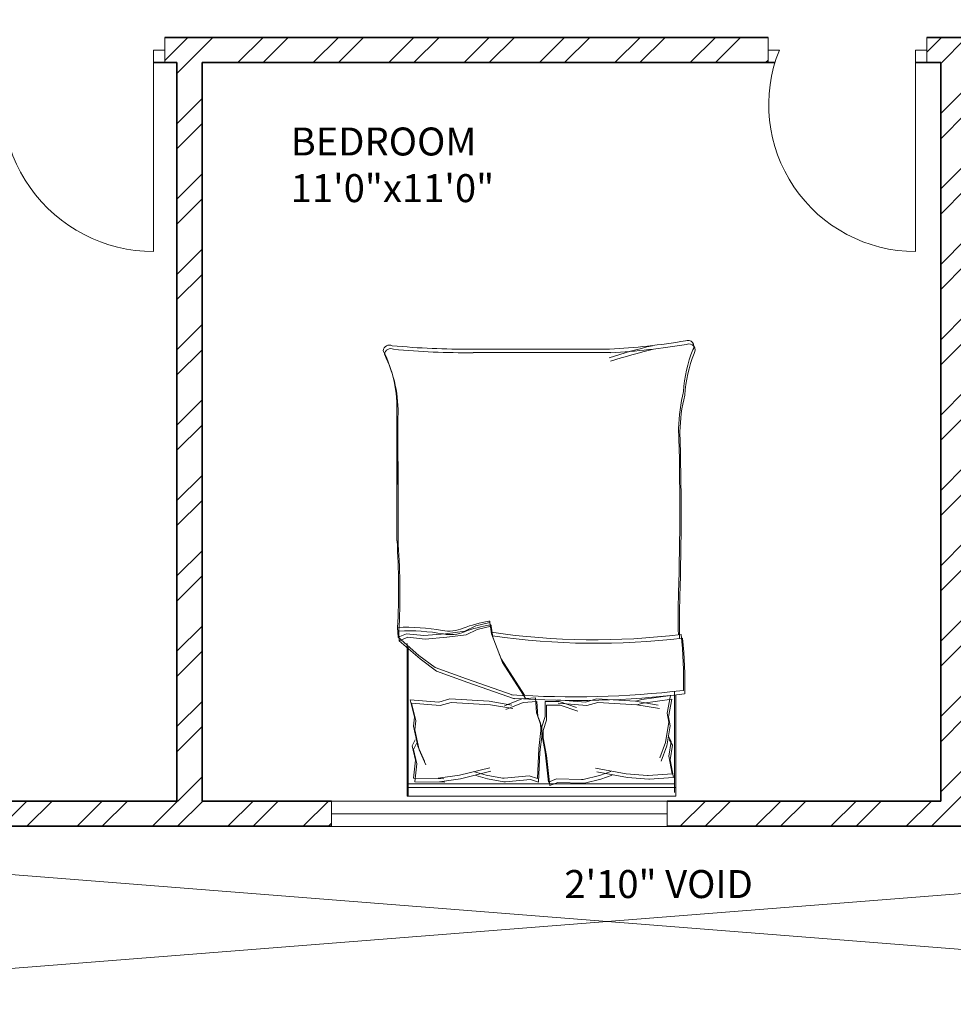
# Model space of a CAD drawing. Units: inches. Extents: x 1885 to 2748, y 783 to 2421.
# Tile 80 of 117: x 2127 to 2294, y 1850 to 2026. Entities that reach past the tile are written whole.
import ezdxf

# ---------------------------------------------------------------- set-up
doc = ezdxf.new("R2010")
doc.units = ezdxf.units.IN
for name, color, linetype, lineweight in [('A-AREA-IDEN', 7, 'Continuous', 18), ('A-DOOR', 31, 'Continuous', 18), ('A-FLOR-OPEN', 8, 'Continuous', 13), ('A-FURN', 8, 'Continuous', 13), ('A-GLAZ', 181, 'Continuous', 18), ('A-WALL', 7, 'Continuous', 35)]:
    doc.layers.add(name, color=color, linetype=linetype, lineweight=lineweight)
doc.layers.add('A-WALL-PATT', color=85, linetype='Continuous', lineweight=13, true_color=0x58ba48)
doc.styles.get("Standard").update_dxf_attribs({"font": 'arial.ttf'})

# ---------------------------------------------------------------- blocks, each defined once
blk = doc.blocks.new('BED-DOUBLE')
for p, q in [((27.75, 52.87), (24.5, 49.16)), ((27.75, 52.87), (24.5, 49.16)), ((28.39, 53.09), (25.14, 49.39)), ((28.39, 53.09), (25.14, 49.39)), ((29.49, 52.95), (27.75, 52.87, 3.87)), ((29.49, 52.95), (27.75, 52.87, 3.87)), ((28.37, 51.33), (27.75, 52.87)), ((28.37, 51.33), (27.75, 52.87)), ((30.13, 53.17), (28.39, 53.09, 3.87)), ((30.13, 53.17), (28.39, 53.09, 3.87)), ((29.01, 51.56), (28.39, 53.09)), ((29.01, 51.56), (28.39, 53.09)), ((0, 51.49), (0.64, 51.49)), ((0, 3.47), (0, 51.49)), ((0, 51.26), (26.61, 51.26)), ((0, 51.26), (26.61, 51.26)), ((0.64, 51.49), (27.25, 51.49)), ((0.64, 51.49), (27.25, 51.49)), ((1.54, 3.47), (1.54, 51.26)), ((1.54, 3.47), (1.54, 51.26)), ((2.18, 3.7), (2.18, 51.49)), ((2.18, 3.7), (2.18, 51.49)), ((28.06, 48.23), (28.37, 51.33)), ((28.06, 48.23), (28.37, 51.33)), ((28.7, 48.46), (29.01, 51.56)), ((28.7, 48.46), (29.01, 51.56)), ((2.56, 50.11), (2.46, 44.71)), ((2.56, 50.11), (2.46, 44.71)), ((2.56, 50.11), (5.77, 49.73)), ((2.56, 50.11), (5.77, 49.73)), ((3.2, 50.34), (3.1, 44.94)), ((3.2, 50.34), (3.1, 44.94)), ((3.2, 50.34), (6.41, 49.96)), ((3.2, 50.34), (6.41, 49.96)), ((8.26, 49.31), (5.58, 48.13)), ((8.26, 49.31), (5.58, 48.13)), ((5.77, 49.73), (8.34, 50.33)), ((5.77, 49.73), (8.34, 50.33)), ((8.9, 49.54), (6.22, 48.36)), ((8.9, 49.54), (6.22, 48.36)), ((6.41, 49.96), (8.98, 50.56)), ((6.41, 49.96), (8.98, 50.56)), ((11.83, 50.11), (8.26, 49.31)), ((11.83, 50.11), (8.26, 49.31)), ((8.34, 50.33), (9.39, 49.81)), ((8.34, 50.33), (9.39, 49.81)), ((12.47, 50.34), (8.9, 49.54)), ((12.47, 50.34), (8.9, 49.54)), ((8.98, 50.56), (10.03, 50.04)), ((8.98, 50.56), (10.03, 50.04)), ((13.44, 49.92), (11.83, 50.11)), ((13.44, 49.92), (11.83, 50.11)), ((14.08, 50.15), (12.47, 50.34)), ((14.08, 50.15), (12.47, 50.34)), ((16.58, 50.7), (13.44, 49.92)), ((16.58, 50.7), (13.44, 49.92)), ((17.22, 50.93), (14.08, 50.15)), ((17.22, 50.93), (14.08, 50.15)), ((16.17, 45.57), (16.58, 50.7)), ((16.17, 45.56), (16.58, 50.7)), ((16.81, 45.79), (17.22, 50.93)), ((16.81, 45.79), (17.22, 50.93)), ((25.14, 49.39), (22.97, 46.45)), ((25.14, 49.39), (22.97, 46.45)), ((24.5, 49.16), (22.33, 46.22)), ((24.5, 49.16), (22.33, 46.22)), ((28.37, 44.36), (28.06, 48.23)), ((28.37, 44.36), (28.06, 48.23)), ((29.01, 44.59), (28.7, 48.46)), ((29.01, 44.59), (28.7, 48.46)), ((3.1, 44.94), (3.19, 45.94)), ((3.1, 44.94), (3.19, 45.94)), ((3.19, 45.94), (3.71, 42.14)), ((3.19, 45.94), (3.71, 42.14)), ((17.37, 43.83), (16.81, 45.79)), ((17.37, 43.83), (16.81, 45.79)), ((22.33, 46.22), (20.32, 40.64)), ((22.33, 46.22), (20.32, 40.64)), ((22.97, 46.45), (20.96, 40.87)), ((22.97, 46.45), (20.96, 40.87)), ((2.46, 44.71), (2.55, 45.71)), ((2.46, 44.71), (2.55, 45.71)), ((2.55, 45.71), (3.07, 41.91)), ((2.55, 45.71), (3.07, 41.91)), ((16.73, 43.6), (16.17, 45.57)), ((16.73, 43.6), (16.17, 45.56)), ((28.83, 40.95), (28.37, 44.36)), ((28.83, 40.95), (28.37, 44.36)), ((29.47, 41.18), (29.01, 44.59)), ((29.47, 41.18), (29.01, 44.59)), ((16.3, 36.59), (16.73, 43.6)), ((16.3, 36.59), (16.73, 43.6)), ((16.94, 36.82), (17.37, 43.83)), ((16.94, 36.82), (17.37, 43.83)), ((3.07, 41.91), (4.43, 36.49)), ((3.07, 41.91), (4.43, 36.49)), ((3.71, 42.14), (5.07, 36.72)), ((3.71, 42.14), (5.07, 36.72)), ((20.32, 40.64), (17.39, 32.3)), ((20.32, 40.64), (17.39, 32.3)), ((20.96, 40.87), (18.03, 32.53)), ((20.96, 40.87), (18.03, 32.53)), ((29.76, 38.94), (28.83, 40.95)), ((29.76, 38.94), (28.83, 40.95)), ((30.4, 39.17), (29.47, 41.18)), ((30.4, 39.17), (29.47, 41.18)), ((3.68, 39.2), (3.08, 37.13)), ((3.68, 39.2), (3.08, 37.13)), ((4.32, 39.43), (3.72, 37.36)), ((4.32, 39.43), (3.72, 37.36)), ((30.38, 36.46), (29.76, 38.94)), ((30.38, 36.46), (29.76, 38.94)), ((31.02, 36.69), (30.4, 39.17)), ((31.02, 36.69), (30.4, 39.17)), ((79.25, 15.06), (79.25, 39.68)), ((79.25, 15.06), (79.25, 39.68)), ((79.89, 15.29), (79.89, 39.9)), ((79.89, 15.29), (79.89, 39.9)), ((3.08, 37.13), (2.54, 34.2)), ((3.08, 37.13), (2.54, 34.2)), ((3.72, 37.36), (3.18, 34.43)), ((3.72, 37.36), (3.18, 34.43)), ((15.63, 32.56), (16.3, 36.59)), ((15.63, 32.56), (16.3, 36.59)), ((16.27, 32.79), (16.94, 36.82)), ((16.27, 32.79), (16.94, 36.82)), ((23.88, 34.45), (28.37, 36.15)), ((23.88, 34.45), (28.37, 36.15)), ((24.52, 34.68), (29.01, 36.38)), ((24.52, 34.68), (29.01, 36.38)), ((28.37, 36.15), (30.38, 36.46)), ((28.37, 36.15), (30.38, 36.46)), ((29.01, 36.38), (31.02, 36.69)), ((29.01, 36.38), (31.02, 36.69)), ((2.54, 34.2), (2.56, 33.88)), ((2.54, 34.2), (2.56, 33.88)), ((2.56, 33.88), (2.98, 29.45)), ((2.56, 33.88), (2.98, 29.45)), ((3.18, 34.43), (3.2, 34.11)), ((3.18, 34.43), (3.2, 34.11)), ((3.2, 34.11), (3.62, 29.68)), ((3.2, 34.11), (3.62, 29.68)), ((16.74, 30.75), (15.46, 33.82)), ((16.74, 30.75), (15.46, 33.82)), ((17.38, 30.98), (16.1, 34.05)), ((17.38, 30.98), (16.1, 34.05)), ((17.39, 30.26), (23.88, 34.45)), ((17.39, 30.26), (23.88, 34.45)), ((18.03, 30.49), (24.52, 34.68)), ((18.03, 30.49), (24.52, 34.68)), ((16.9, 28.3), (16.74, 30.75)), ((16.9, 28.3), (16.74, 30.75)), ((17.54, 28.52), (17.38, 30.98)), ((17.54, 28.52), (17.38, 30.98)), ((2.98, 29.45), (2.5, 27.98)), ((2.98, 29.45), (2.5, 27.98)), ((3.62, 29.68), (3.13, 28.2)), ((3.62, 29.68), (3.13, 28.2)), ((3.13, 28.2), (8.51, 27.96)), ((3.13, 28.2), (8.51, 27.96)), ((13.02, 27.66), (14.86, 28.36)), ((13.02, 27.66), (14.86, 28.36)), ((14.22, 28.13), (16.9, 28.3)), ((14.22, 28.13), (16.9, 28.3)), ((14.86, 28.36), (17.54, 28.52)), ((14.86, 28.36), (17.54, 28.52)), ((1.87, 25.98), (7.22, 26.56)), ((1.87, 25.98), (7.22, 26.56)), ((2.5, 27.98), (7.87, 27.73)), ((2.5, 27.98), (7.87, 27.73)), ((2.51, 26.21), (7.86, 26.79)), ((2.51, 26.21), (7.86, 26.79)), ((7.22, 26.56), (10.4, 27.14)), ((7.22, 26.56), (10.4, 27.14)), ((7.86, 26.79), (11.04, 27.37)), ((7.86, 26.79), (11.04, 27.37)), ((7.87, 27.73), (11.08, 27.35)), ((7.87, 27.73), (11.08, 27.35)), ((8.51, 27.96), (11.72, 27.58)), ((8.51, 27.96), (11.72, 27.58)), ((10.4, 27.14), (11.71, 27.14)), ((10.4, 27.14), (11.71, 27.14)), ((11.04, 27.37), (12.35, 27.37)), ((11.04, 27.37), (12.35, 27.37)), ((11.08, 27.35), (12.38, 27.43)), ((11.08, 27.35), (12.38, 27.43)), ((11.71, 27.14), (13.59, 26.56)), ((11.71, 27.14), (13.59, 26.56)), ((11.72, 27.58), (13.02, 27.66)), ((11.72, 27.58), (13.02, 27.66)), ((12.35, 27.37), (14.22, 26.79)), ((12.35, 27.37), (14.22, 26.79)), ((12.38, 27.43), (14.22, 28.13)), ((12.38, 27.43), (14.22, 28.13)), ((13.59, 26.56), (16.27, 26.56)), ((13.59, 26.56), (16.27, 26.56)), ((14.22, 26.79), (16.91, 26.79)), ((14.22, 26.79), (16.91, 26.79)), ((16.27, 26.56), (16.27, 24.1)), ((16.27, 26.56), (16.27, 24.1)), ((16.91, 26.79), (16.91, 24.33)), ((16.91, 26.79), (16.91, 24.33)), ((2.45, 24.54), (1.87, 25.98)), ((2.45, 24.54), (1.87, 25.98)), ((3.09, 24.76), (2.51, 26.21)), ((3.09, 24.76), (2.51, 26.21)), ((2.95, 20.32), (3.09, 24.76)), ((2.95, 20.32), (3.09, 24.76)), ((16.81, 19.61), (17.22, 24.74)), ((16.81, 19.61), (17.22, 24.74)), ((2.31, 20.09), (2.45, 24.54)), ((2.31, 20.09), (2.45, 24.54)), ((16.27, 24.1), (15.18, 20.96)), ((16.27, 24.1), (15.18, 20.96)), ((16.91, 24.33), (15.82, 21.19)), ((16.91, 24.33), (15.82, 21.19)), ((16.17, 19.38), (16.58, 24.51)), ((16.17, 19.38), (16.58, 24.51)), ((2.31, 19.77), (2.31, 20.09)), ((2.31, 19.77), (2.31, 20.09)), ((3.03, 16.88), (2.31, 19.77)), ((3.03, 16.88), (2.31, 19.77)), ((2.95, 20), (2.95, 20.32)), ((2.95, 20), (2.95, 20.32)), ((3.67, 17.11), (2.95, 20)), ((3.67, 17.11), (2.95, 20)), ((16.73, 17.42), (16.17, 19.38)), ((16.73, 17.42), (16.17, 19.38)), ((17.37, 17.65), (16.81, 19.61)), ((17.37, 17.65), (16.81, 19.61)), ((3.32, 12.11), (4.33, 17.6)), ((3.32, 12.11), (4.33, 17.6)), ((3.96, 12.34), (4.97, 17.83)), ((3.96, 12.34), (4.97, 17.83)), ((16.94, 10.64), (17.37, 17.65)), ((16.94, 10.64), (17.37, 17.65)), ((3.75, 14.85), (3.03, 16.88)), ((3.75, 14.85), (3.03, 16.88)), ((4.39, 15.08), (3.67, 17.11)), ((4.39, 15.08), (3.67, 17.11)), ((16.3, 10.41), (16.73, 17.42)), ((16.3, 10.41), (16.73, 17.42)), ((3.67, 8.51), (3.96, 12.34)), ((3.67, 8.51), (3.96, 12.34)), ((3.03, 8.28), (3.32, 12.11)), ((3.03, 8.28), (3.32, 12.11)), ((16.27, 6.61), (16.94, 10.64)), ((16.27, 6.61), (16.94, 10.64)), ((16.94, 10.64), (17.26, 9.51)), ((16.94, 10.64), (17.26, 9.51)), ((15.63, 6.38), (16.3, 10.41)), ((15.63, 6.38), (16.3, 10.41)), ((16.3, 10.41), (16.62, 9.28)), ((16.3, 10.41), (16.62, 9.28)), ((16.62, 9.28), (17.34, 4.18)), ((16.62, 9.28), (17.34, 4.18)), ((17.26, 9.51), (17.98, 4.41)), ((17.26, 9.51), (17.98, 4.41)), ((3.01, 8.18), (3.03, 8.28)), ((3.01, 8.18), (3.03, 8.28)), ((3.34, 3.9), (3.01, 8.18)), ((3.34, 3.9), (3.01, 8.18)), ((3.65, 8.41), (3.67, 8.51)), ((3.65, 8.41), (3.67, 8.51)), ((3.98, 4.13), (3.65, 8.41)), ((3.98, 4.13), (3.65, 8.41)), ((8.96, 5.05), (6.21, 6.06)), ((8.96, 5.05), (6.21, 6.06)), ((9.6, 5.28), (6.85, 6.29)), ((9.6, 5.28), (6.85, 6.29)), ((18.75, 3.7), (0.64, 3.7)), ((18.75, 3.7), (0.64, 3.7)), ((3.32, 3.89), (6.5, 4.47)), ((3.32, 3.89), (6.5, 4.47)), ((3.96, 4.12), (7.14, 4.7)), ((3.96, 4.12), (7.14, 4.7)), ((6.5, 4.47), (9.1, 4.04)), ((6.5, 4.47), (9.1, 4.04)), ((7.14, 4.7), (9.74, 4.27)), ((7.14, 4.7), (9.74, 4.27)), ((12.57, 4.47), (8.96, 5.05)), ((12.57, 4.47), (8.96, 5.05)), ((9.1, 4.04), (10.12, 4.62)), ((9.1, 4.04), (10.12, 4.62)), ((13.21, 4.7), (9.6, 5.28)), ((13.21, 4.7), (9.6, 5.28)), ((9.74, 4.27), (10.75, 4.84)), ((9.74, 4.27), (10.75, 4.84)), ((14.16, 4.76), (12.57, 4.47)), ((14.16, 4.76), (12.57, 4.47)), ((14.8, 4.99), (13.21, 4.7)), ((14.8, 4.99), (13.21, 4.7)), ((17.34, 4.18), (14.16, 4.76)), ((17.34, 4.18), (14.16, 4.76)), ((17.98, 4.41), (14.8, 4.99)), ((17.98, 4.41), (14.8, 4.99)), ((18.11, 3.47), (0, 3.47)), ((18.11, 3.47), (0, 3.47))]:
    blk.add_line(p, q)
for centre, radius, start, end in [((68.67, 76.16), 23.07, 267.4714, 296.4681), ((68.67, 76.16), 23.07, 267.4714, 296.4681), ((69.31, 76.38), 23.07, 267.4714, 296.4681), ((69.31, 76.38), 23.07, 267.4714, 296.4681), ((78.87, 54.41), 1.1, 332.6588, 86.02), ((78.87, 54.41), 1.1, 332.6588, 86.02), ((79.51, 54.64), 1.1, 332.6588, 86.02), ((79.51, 54.64), 1.1, 332.6588, 86.02), ((-6.65, 51.33), 36.18, 349.8763, 2.5657), ((-6.65, 51.33), 36.18, 349.8763, 2.5657), ((36.32, 182.26), 129.5, 266.9791, 273.8365), ((36.32, 182.26), 129.5, 266.9791, 273.8365), ((-6.01, 51.55), 36.18, 349.8763, 2.5657), ((-6.01, 51.55), 36.18, 349.8763, 2.5657), ((36.96, 182.49), 129.5, 266.9791, 273.8365), ((36.96, 182.49), 129.5, 266.9791, 273.8365), ((67.83, -4508.74), 4561.86, 90.00217, 90.28689), ((67.83, -4508.75), 4561.86, 90.00217, 90.28689), ((68.46, -4508.52), 4561.86, 90.00217, 90.28689), ((68.46, -4508.52), 4561.86, 90.00217, 90.28689), ((212.28, 41.15), 133.04, 174.4998, 180.6351), ((212.28, 41.15), 133.04, 174.4998, 180.6351), ((212.92, 41.38), 133.04, 174.4998, 180.6351), ((212.92, 41.38), 133.04, 174.4998, 180.6351), ((35.07, 43.74), 6.22, 168.6608, 203.7384), ((35.07, 43.74), 6.22, 168.6608, 203.7384), ((35.71, 43.97), 6.22, 168.6608, 203.7384), ((35.71, 43.97), 6.22, 168.6608, 203.7384), ((1.49, 31.15), 29.65, 10.6617, 19.8806), ((1.49, 31.15), 29.65, 10.6617, 19.8806), ((2.13, 31.38), 29.65, 10.6617, 19.8806), ((2.13, 31.38), 29.65, 10.6617, 19.8806), ((156.32, 17.75), 129.02, 171.7845, 186.9006), ((156.32, 17.75), 129.02, 171.7845, 186.9006), ((156.96, 17.98), 129.02, 171.7845, 186.9006), ((156.96, 17.98), 129.02, 171.7845, 186.9006), ((30.44, 36.64), 0.185, 250.2464, 1.1377), ((30.44, 36.63), 0.185, 250.2464, 1.1377), ((31.08, 36.86), 0.185, 250.2464, 1.1377), ((31.08, 36.86), 0.185, 250.2464, 1.1377), ((182.06, 21.36), 164.97, 176.0865, 186.7821), ((182.06, 21.36), 164.97, 176.0865, 186.7821), ((182.7, 21.59), 164.97, 176.0865, 186.7821), ((182.7, 21.59), 164.97, 176.0865, 186.7821), ((-23.71, -17.22), 106.46, 13.3832, 17.7053), ((-23.71, -17.22), 106.46, 13.3832, 17.7053), ((-23.07, -16.99), 106.46, 13.3832, 17.7053), ((-23.07, -16.99), 106.46, 13.3832, 17.7053), ((200.84, 21.43), 121.76, 182.9958, 189.4091), ((200.84, 21.43), 121.76, 182.9958, 189.4091), ((201.48, 21.65), 121.76, 182.9958, 189.4091), ((201.48, 21.65), 121.76, 182.9958, 189.4091), ((20.1, 85.16), 83.31, 268.7218, 275.604), ((20.1, 85.16), 83.31, 268.7218, 275.604), ((20.74, 85.39), 83.31, 268.7218, 275.604), ((20.74, 85.39), 83.31, 268.7218, 275.604), ((31.18, -167.31), 170.11, 88.4762, 91.0082), ((31.18, -167.31), 170.11, 88.4762, 91.0082), ((31.82, -167.08), 170.11, 88.4762, 91.0082), ((31.82, -167.08), 170.11, 88.4762, 91.0082), ((50.62, 484.82), 482.31, 268.2277, 271.7185), ((50.62, 484.82), 482.31, 268.2277, 271.7185), ((51.26, 485.05), 482.31, 268.2277, 271.7185), ((51.26, 485.05), 482.31, 268.2277, 271.7185), ((64.52, -26.9), 29.63, 76.0648, 88.9113), ((64.52, -26.9), 29.63, 76.0648, 88.9113), ((65.16, -26.67), 29.63, 76.0648, 88.9113), ((65.16, -26.67), 29.63, 76.0648, 88.9113), ((70.28, -21.66), 23.56, 67.9751, 86.652), ((70.28, -21.66), 23.56, 67.9751, 86.652), ((70.92, -21.43), 23.56, 67.9751, 86.652), ((70.92, -21.43), 23.56, 67.9751, 86.652), ((79.72, 1.09), 1.09, 236.1736, 23.4781), ((79.72, 1.09), 1.09, 236.1736, 23.4781), ((80.36, 1.31), 1.09, 236.1736, 23.4781), ((80.36, 1.31), 1.09, 236.1736, 23.4781)]:
    blk.add_arc(centre, radius, start, end)
blk = doc.blocks.new('WIN-60')
for p, q in [((0, 60), (4.5, 60)), ((0, 60), (0, 0)), ((4.5, 60), (2.25, 60)), ((2.25, 60), (2.25, 0)), ((4.5, 0), (4.5, 60)), ((2.25, 0), (0, 0)), ((0, 0), (4.5, 0))]:
    blk.add_line(p, q)

msp = doc.modelspace()

# ---------------------------------------------------------------- hatches: boundary and pattern name
at = {"layer": 'A-WALL-PATT'}
h = msp.add_hatch(dxfattribs=at)
h.set_pattern_fill('ANSI32', color=256)
h.paths.add_polyline_path([(2007.77, 2318.01), (1980.77, 2318.01), (1980.77, 2281.22), (1985.27, 2281.22), (1985.27, 2313.51), (2007.77, 2313.51), (2007.77, 2315.76)])
h.paths.add_polyline_path([(2094.32, 2318.01), (2067.77, 2318.01), (2067.77, 2313.51), (2094.32, 2313.51), (2094.32, 2315.76)])
h.paths.add_polyline_path([(2131.37, 2315.76), (2131.37, 2318.01), (2131.19, 2318.01), (2112.61, 2318.01), (2112.61, 2313.51), (2117.27, 2313.51), (2117.27, 2255.2), (2121.77, 2255.2), (2121.77, 2313.51), (2131.37, 2313.51)])
h.paths.add_polyline_path([(2190.51, 2318.01), (2155.37, 2318.01), (2155.37, 2313.51), (2169.77, 2313.51), (2169.77, 2229.51), (2121.77, 2229.51), (2121.77, 2233.45), (2119.52, 2233.45), (2117.27, 2233.45), (2117.27, 2201.1), (2121.77, 2201.1), (2121.77, 2225.01), (2169.77, 2225.01), (2169.77, 2165.01), (2306.27, 2165.01), (2306.27, 2066.01), (2310.77, 2066.01), (2344.27, 2066.01), (2486.27, 2066.01), (2486.27, 1886.01), (2483.02, 1886.01), (2483.02, 1881.51), (2486.27, 1881.51), (2486.27, 1880.68), (2490.77, 1880.68), (2490.77, 2070.51), (2344.27, 2070.51), (2310.77, 2070.51), (2310.77, 2165.01), (2310.77, 2173.64), (2308.52, 2173.64), (2306.27, 2173.64), (2306.27, 2169.51), (2174.27, 2169.51), (2174.27, 2313.51), (2190.51, 2313.51), (2190.51, 2315.76)])
h.paths.add_polyline_path([(1985.27, 2221.22), (1980.77, 2221.22), (1980.77, 2165.01), (1992.77, 2165.01), (1992.77, 2141.93), (1997.27, 2141.93), (1997.27, 2165.01), (2117.27, 2165.01), (2117.27, 2163.13), (2121.77, 2163.13), (2121.77, 2172.73), (2119.52, 2172.73), (2117.27, 2172.73), (2117.27, 2169.51), (1985.27, 2169.51)])
h.paths.add_polyline_path([(1997.27, 2105.93), (1992.77, 2105.93), (1992.77, 2070.51), (2016.77, 2070.51), (2016.77, 2059.12), (2019.02, 2059.12), (2021.27, 2059.12), (2021.27, 2070.51), (2117.27, 2070.51), (2117.27, 2022.51), (2114.42, 2022.51), (2114.42, 2018.01), (2123.63, 2018.01), (2123.63, 2020.26), (2123.63, 2022.51), (2121.77, 2022.51), (2121.77, 2142.59), (2119.52, 2142.59), (2117.27, 2142.59), (2117.27, 2075.01), (1997.27, 2075.01)])
h.paths.add_polyline_path([(2092.03, 2020.26), (2092.03, 2022.51), (2021.27, 2022.51), (2021.27, 2035.12), (2016.77, 2035.12), (2016.77, 2018.01), (2016.77, 1978.78), (2021.27, 1978.78), (2021.27, 2018.01), (2092.03, 2018.01)])
h.paths.add_polyline_path([(2260.94, 2022.51), (2153.1, 2022.51), (2153.1, 2020.26), (2153.1, 2018.01), (2155.27, 2018.01), (2155.27, 1886.01), (2107.63, 1886.01), (2107.63, 1881.51), (2182.91, 1881.51), (2182.91, 1883.76), (2182.91, 1886.01), (2159.77, 1886.01), (2159.77, 2018.01), (2260.94, 2018.01), (2260.94, 2020.26)])
h.paths.add_polyline_path([(2047.63, 1883.76), (2047.63, 1886.01), (2021.27, 1886.01), (2021.27, 1918.78), (2019.02, 1918.78), (2016.77, 1918.78), (2016.77, 1881.51), (2047.63, 1881.51)])
h.paths.add_polyline_path([(2306.36, 1883.76), (2306.36, 1886.01), (2296.27, 1886.01), (2296.27, 1982.01), (2316.54, 1982.01), (2316.54, 1984.26), (2316.54, 1986.51), (2296.27, 1986.51), (2296.27, 2022.51), (2289.28, 2022.51), (2289.28, 2018.01), (2291.77, 2018.01), (2291.77, 1886.01), (2242.91, 1886.01), (2242.91, 1881.51), (2306.36, 1881.51)], flags=17)
h.paths.add_polyline_path([(1985.27, 1843.01), (2021.6, 1843.01), (2021.53, 1845.44), (2021.48, 1847.51), (1980.77, 1847.51), (1980.77, 1809.45), (1985.27, 1809.45)])
h.paths.add_polyline_path([(2131.48, 1845.26), (2131.48, 1847.51), (2081.53, 1847.51), (2081.53, 1843.01), (2117.27, 1843.01), (2117.27, 1784.15), (2119.52, 1784.15), (2121.77, 1784.15), (2121.77, 1843.01), (2131.48, 1843.01)])
h.paths.add_polyline_path([(2203.89, 1847.51), (2155.48, 1847.51), (2155.48, 1843.01), (2169.77, 1843.01), (2169.77, 1759.01), (2121.77, 1759.01), (2121.77, 1761.46), (2117.27, 1761.46), (2117.27, 1730.43), (2121.77, 1730.43), (2121.77, 1754.51), (2177.42, 1754.51), (2177.42, 1756.76), (2177.42, 1759.01), (2174.27, 1759.01), (2174.27, 1843.01), (2203.89, 1843.01)])
h.paths.add_polyline_path([(2335.55, 1845.26), (2335.55, 1847.51), (2239.89, 1847.51), (2239.89, 1843.01), (2306.27, 1843.01), (2306.27, 1759.01), (2199.49, 1759.01), (2199.49, 1754.51), (2310.77, 1754.51), (2310.77, 1843.01), (2335.55, 1843.01)])
h.paths.add_polyline_path([(2348.77, 2022.51), (2344.27, 2022.51), (2344.27, 1986.51), (2341.68, 1986.51), (2341.68, 1982.01), (2344.27, 1982.01), (2344.27, 1886.01), (2330.36, 1886.01), (2330.36, 1881.51), (2361.63, 1881.51), (2361.63, 1883.76), (2361.63, 1886.01), (2348.77, 1886.01)], flags=17)
h.paths.add_polyline_path([(2283.25, 2315.76), (2283.25, 2318.01), (2238.51, 2318.01), (2238.51, 2313.51), (2283.25, 2313.51)], flags=17)
h.paths.add_polyline_path([(2363.27, 2348.01), (2388.68, 2348.01), (2388.68, 2350.26), (2388.68, 2352.51), (2358.77, 2352.51), (2358.77, 2348.01), (2358.77, 2318.01), (2344.48, 2318.01), (2344.48, 2313.51), (2358.77, 2313.51), (2358.77, 2229.51), (2310.77, 2229.51), (2310.77, 2231.95), (2306.27, 2231.95), (2306.27, 2205.61), (2310.77, 2205.61), (2310.77, 2225.01), (2358.77, 2225.01), (2358.77, 2211.51), (2452.33, 2211.51), (2452.33, 2213.76), (2452.33, 2216.01), (2363.27, 2216.01), (2363.27, 2318.01)])
h.paths.add_polyline_path([(2310.77, 2313.51), (2320.48, 2313.51), (2320.48, 2315.76), (2320.48, 2318.01), (2302.73, 2318.01), (2302.73, 2313.51), (2306.27, 2313.51), (2306.27, 2251.08), (2310.77, 2251.08)], flags=17)
h.paths.add_polyline_path([(2490.77, 2352.51), (2486.27, 2352.51), (2448.68, 2352.51), (2448.68, 2348.01), (2486.27, 2348.01), (2486.27, 2318.01), (2486.27, 2216.01), (2481.78, 2216.01), (2481.78, 2211.51), (2486.27, 2211.51), (2486.27, 2165.01), (2493.29, 2165.01), (2493.29, 2167.26), (2493.29, 2169.51), (2490.77, 2169.51), (2490.77, 2313.51), (2494.43, 2313.51), (2494.43, 2318.01), (2490.77, 2318.01)])
h.paths.add_polyline_path([(2534.65, 2318.01), (2515.69, 2318.01), (2515.69, 2313.51), (2534.65, 2313.51), (2534.65, 2315.76)])
h.paths.add_polyline_path([(2618.27, 2318.01), (2594.65, 2318.01), (2594.65, 2313.51), (2613.77, 2313.51), (2613.77, 2281.71), (2618.27, 2281.71)])
h.paths.add_polyline_path([(2618.27, 2221.71), (2613.77, 2221.71), (2613.77, 2169.51), (2554.02, 2169.51), (2554.02, 2165.01), (2613.77, 2165.01), (2613.77, 2152.88), (2618.27, 2152.88)])
h.paths.add_polyline_path([(2618.27, 2128.88), (2616.02, 2128.88), (2613.77, 2128.88), (2613.77, 2117.01), (2529.77, 2117.01), (2529.77, 2165.01), (2532.85, 2165.01), (2532.85, 2169.51), (2522.87, 2169.51), (2522.87, 2165.01), (2525.27, 2165.01), (2525.27, 2117.01), (2525.27, 2112.51), (2525.27, 2108.58), (2529.77, 2108.58), (2529.77, 2112.51), (2613.77, 2112.51), (2613.77, 2080.19), (2618.27, 2080.19)])
h.paths.add_polyline_path([(2618.27, 2044.19), (2616.02, 2044.19), (2613.77, 2044.19), (2613.77, 2015.51), (2529.77, 2015.51), (2529.77, 2088.58), (2527.52, 2088.58), (2525.27, 2088.58), (2525.27, 2011.01), (2613.77, 2011.01), (2613.77, 1956.75), (2618.27, 1956.75)])
h.paths.add_polyline_path([(2618.27, 1881.51), (2618.27, 1896.75), (2613.77, 1896.75), (2613.77, 1881.51), (2613.77, 1847.51), (2592.71, 1847.51), (2592.71, 1843.01), (2613.77, 1843.01), (2613.77, 1765.01), (2613.77, 1760.51), (2609.62, 1760.51), (2609.62, 1756.01), (2613.77, 1756.01), (2613.77, 1660.01), (2608.54, 1660.01), (2608.54, 1655.51), (2613.77, 1655.51), (2613.77, 1508.16), (2618.27, 1508.16)])
h.paths.add_polyline_path([(2565.77, 1843.01), (2569, 1843.01), (2569, 1847.51), (2490.77, 1847.51), (2490.77, 1849.7), (2488.52, 1849.7), (2486.27, 1849.7), (2486.27, 1847.51), (2477.27, 1847.51), (2477.27, 1838.51), (2477.27, 1821.49), (2486.27, 1821.49), (2486.27, 1838.51), (2561.27, 1838.51), (2561.27, 1765.01), (2486.27, 1765.01), (2486.27, 1786.16), (2477.27, 1786.16), (2477.27, 1765.01), (2477.27, 1756.01), (2486.27, 1756.01), (2565.77, 1756.01), (2585.62, 1756.01), (2585.62, 1758.26), (2585.62, 1760.51), (2565.77, 1760.51), (2565.77, 1765.01)])
h.paths.add_polyline_path([(2486.27, 1651.01), (2561.27, 1651.01), (2561.27, 1567.01), (2486.27, 1567.01), (2486.27, 1591.32), (2477.27, 1591.32), (2477.27, 1567.01), (2477.27, 1558.01), (2477.27, 1555.44), (2481.77, 1555.44), (2481.77, 1558.01), (2568.65, 1558.01), (2568.65, 1560.26), (2568.65, 1562.51), (2565.77, 1562.51), (2565.77, 1655.51), (2584.54, 1655.51), (2584.54, 1657.76), (2584.54, 1660.01), (2565.77, 1660.01), (2486.27, 1660.01), (2477.27, 1660.01), (2477.27, 1651.01), (2477.27, 1632.99), (2486.27, 1632.99)])
h.paths.add_polyline_path([(2449.97, 1883.76), (2449.97, 1886.01), (2421.63, 1886.01), (2421.63, 1881.51), (2449.97, 1881.51)], flags=17)
h.paths.add_polyline_path([(2447.27, 1847.51), (2395.55, 1847.51), (2395.55, 1843.01), (2442.77, 1843.01), (2442.77, 1809.27), (2447.27, 1809.27)])
h.paths.add_polyline_path([(1985.27, 1749.45), (1980.77, 1749.45), (1980.77, 1694.5), (1985.27, 1694.5), (1985.27, 1694.51), (1986.9, 1694.51), (1986.9, 1697.78), (1986.9, 1699.01), (1985.27, 1699.01)])
h.paths.add_polyline_path([(2152.77, 1699.01), (2121.77, 1699.01), (2121.77, 1703.67), (2119.52, 1703.67), (2117.27, 1703.67), (2117.27, 1699.01), (2009.22, 1699.01), (2009.22, 1694.51), (2148.27, 1694.51), (2148.27, 1692.63), (2152.77, 1692.63)])
h.paths.add_polyline_path([(2016.27, 1694.51), (2011.77, 1694.51), (2011.77, 1558.01), (2040.81, 1558.01), (2040.81, 1560.26), (2040.81, 1562.51), (2016.27, 1562.51)])
h.paths.add_polyline_path([(2152.77, 1663.02), (2150.52, 1663.02), (2148.27, 1663.02), (2148.27, 1562.51), (2100.81, 1562.51), (2100.81, 1558.01), (2165.12, 1558.01), (2165.12, 1560.26), (2165.12, 1562.51), (2152.77, 1562.51), (2152.77, 1610.51), (2224.77, 1610.51), (2224.77, 1607.99), (2229.27, 1607.99), (2229.27, 1615.01), (2152.77, 1615.01)])
h.paths.add_polyline_path([(2238.61, 1560.26), (2238.61, 1562.51), (2229.27, 1562.51), (2229.27, 1588.76), (2227.02, 1588.76), (2224.77, 1588.77), (2224.77, 1562.51), (2189.12, 1562.51), (2189.12, 1558.01), (2238.61, 1558.01)])
h.paths.add_polyline_path([(2336.02, 1560.26), (2336.02, 1562.51), (2310.77, 1562.51), (2310.77, 1656.35), (2308.52, 1656.35), (2306.27, 1656.35), (2306.27, 1562.51), (2286.61, 1562.51), (2286.61, 1558.01), (2336.02, 1558.01)])
h.paths.add_polyline_path([(2447.27, 1690.97), (2445.02, 1690.97), (2442.77, 1690.97), (2442.77, 1687.01), (2306.27, 1687.01), (2306.27, 1680.75), (2310.77, 1680.75), (2310.77, 1682.51), (2442.77, 1682.51), (2442.77, 1562.51), (2396.02, 1562.51), (2396.02, 1558.01), (2447.27, 1558.01)])
h.paths.add_polyline_path([(2447.27, 1749.27), (2445.02, 1749.27), (2442.77, 1749.27), (2442.77, 1717.23), (2447.27, 1717.23)])
h.paths.add_polyline_path([(2044.67, 1521.76), (2044.67, 1524.01), (2007.27, 1524.01), (2007.27, 1503.49), (2009.52, 1503.49), (2011.77, 1503.49), (2011.77, 1519.51), (2044.67, 1519.51)])
h.paths.add_polyline_path([(2177.97, 1521.76), (2177.97, 1524.01), (2104.67, 1524.01), (2104.67, 1519.51), (2145.77, 1519.51), (2145.77, 1387.51), (2143.37, 1387.51), (2143.37, 1383.01), (2251.59, 1383.01), (2251.59, 1385.26), (2251.59, 1387.51), (2150.27, 1387.51), (2150.27, 1519.51), (2177.97, 1519.51)])
h.paths.add_polyline_path([(2298.7, 1524.01), (2237.97, 1524.01), (2237.97, 1519.51), (2282.27, 1519.51), (2282.27, 1387.51), (2279.68, 1387.51), (2279.68, 1383.01), (2286.77, 1383.01), (2286.77, 1419.01), (2312.45, 1419.01), (2312.45, 1421.26), (2312.45, 1423.51), (2286.77, 1423.51), (2286.77, 1519.51), (2298.7, 1519.51), (2298.7, 1521.72)], flags=17)
h.paths.add_polyline_path([(2361.9, 1521.76), (2361.9, 1524.01), (2322.7, 1524.01), (2322.7, 1519.51), (2334.77, 1519.51), (2334.77, 1423.51), (2331.93, 1423.51), (2331.93, 1419.01), (2334.77, 1419.01), (2334.77, 1387.51), (2334.77, 1383.23), (2339.27, 1383.23), (2339.27, 1387.51), (2339.27, 1519.51), (2361.9, 1519.51)], flags=17)
h.paths.add_polyline_path([(2447.27, 1521.76), (2447.27, 1524.01), (2421.9, 1524.01), (2421.9, 1519.51), (2447.27, 1519.51)], flags=17)
h.paths.add_polyline_path([(2481.77, 1529.6), (2479.52, 1529.6), (2477.27, 1529.6), (2477.27, 1524.01), (2474.49, 1524.01), (2474.49, 1519.51), (2477.27, 1519.51), (2477.27, 1334.51), (2296.77, 1334.51), (2296.77, 1240.51), (2160.27, 1240.51), (2160.27, 1180.51), (2112.27, 1180.51), (2112.27, 1207.69), (2110.02, 1207.69), (2107.77, 1207.69), (2107.77, 1171.61), (2112.27, 1171.61), (2112.27, 1176.01), (2160.27, 1176.01), (2160.27, 1092.01), (2144.22, 1092.01), (2144.22, 1087.51), (2189.5, 1087.51), (2189.5, 1089.76), (2189.5, 1092.01), (2164.77, 1092.01), (2164.77, 1236.01), (2296.77, 1236.01), (2296.77, 1231.91), (2301.27, 1231.91), (2301.27, 1330.01), (2481.77, 1330.01), (2481.77, 1387.51)])
h.paths.add_polyline_path([(2618.27, 1448.16), (2613.77, 1448.16), (2613.77, 1382.51), (2529.77, 1382.51), (2525.27, 1382.51), (2525.27, 1307.06), (2529.77, 1307.06), (2529.77, 1378.01), (2613.77, 1378.01), (2613.77, 1354.99), (2618.27, 1354.99)])
h.paths.add_polyline_path([(2618.27, 1318.99), (2613.77, 1318.99), (2613.77, 1281.01), (2529.77, 1281.01), (2529.77, 1283.79), (2527.52, 1283.79), (2525.27, 1283.79), (2525.27, 1228.51), (2516.79, 1228.51), (2516.79, 1224.01), (2533.48, 1224.01), (2533.48, 1226.26), (2533.48, 1228.51), (2529.77, 1228.51), (2529.77, 1276.51), (2613.77, 1276.51), (2613.77, 1266.02), (2618.27, 1266.02)])
h.paths.add_polyline_path([(2618.27, 1134.96), (2613.77, 1134.96), (2613.77, 1092.01), (2594.54, 1092.01), (2594.54, 1087.51), (2618.27, 1087.51)])
h.paths.add_polyline_path([(2534.54, 1092.01), (2509.77, 1092.01), (2509.77, 1087.51), (2534.54, 1087.51), (2534.54, 1089.76)])
h.paths.add_polyline_path([(2481.27, 1224.01), (2484.12, 1224.01), (2484.12, 1226.26), (2484.12, 1228.51), (2476.77, 1228.51), (2476.77, 1198.51), (2471.61, 1198.51), (2471.61, 1194.01), (2476.77, 1194.01), (2476.77, 1062.01), (2436.89, 1062.01), (2436.89, 1057.51), (2476.77, 1057.51), (2481.27, 1057.51), (2481.27, 1062.01), (2481.27, 1087.51), (2485.35, 1087.51), (2485.35, 1089.76), (2485.35, 1092.01), (2481.27, 1092.01), (2481.27, 1117.51)])
h.paths.add_polyline_path([(2439.9, 1198.51), (2349.27, 1198.51), (2349.27, 1194.01), (2349.27, 1180.51), (2301.27, 1180.51), (2301.27, 1201.9), (2299.02, 1201.9), (2296.77, 1201.9), (2296.77, 1172.34), (2299.02, 1172.34), (2301.27, 1172.34), (2301.27, 1176.01), (2349.27, 1176.01), (2349.27, 1092.01), (2334.45, 1092.01), (2334.45, 1087.51), (2349.27, 1087.51), (2349.27, 1057.51), (2353.77, 1057.51), (2376.89, 1057.51), (2376.89, 1059.76), (2376.89, 1062.01), (2353.77, 1062.01), (2353.77, 1087.51), (2353.77, 1180.51), (2353.77, 1194.01), (2439.9, 1194.01), (2439.9, 1196.26)])
h.paths.add_polyline_path([(2270.6, 1089.76), (2270.6, 1092.01), (2249.5, 1092.01), (2249.5, 1087.51), (2270.6, 1087.51)], flags=17)
h.paths.add_polyline_path([(2310.45, 1092.01), (2301.27, 1092.01), (2301.27, 1153.29), (2296.77, 1153.29), (2296.77, 1092.01), (2293.79, 1092.01), (2293.79, 1087.51), (2310.45, 1087.51), (2310.45, 1089.76)], flags=17)
h.paths.add_polyline_path([(2112.27, 1150.33), (2110.02, 1150.33), (2107.77, 1150.33), (2107.77, 1092.01), (2104.47, 1092.01), (2104.47, 1087.51), (2120.22, 1087.51), (2120.22, 1089.76), (2120.22, 1092.01), (2112.27, 1092.01)])
h.paths.add_polyline_path([(2082.17, 1092.01), (2058.14, 1092.01), (2058.14, 1087.51), (2082.17, 1087.51), (2082.17, 1089.76)])
h.paths.add_polyline_path([(1975.77, 1145.64), (1971.27, 1145.64), (1971.27, 1087.51), (1980.77, 1087.51), (1998.14, 1087.51), (1998.14, 1089.76), (1998.14, 1092.01), (1985.27, 1092.01), (1975.77, 1092.01)])
h.paths.add_polyline_path([(2112.27, 1244.38), (2110.02, 1244.38), (2107.77, 1244.38), (2107.77, 1240.51), (1992.27, 1240.51), (1992.27, 1271.01), (1987.77, 1271.01), (1987.77, 1240.51), (1980.77, 1240.51), (1975.77, 1240.51), (1971.27, 1240.51), (1971.27, 1205.64), (1975.77, 1205.64), (1975.77, 1236.01), (2107.77, 1236.01), (2107.77, 1233.44), (2112.27, 1233.44), (2112.27, 1236.01)])
h.paths.add_polyline_path([(2112.27, 1383.01), (2114.78, 1383.01), (2114.78, 1385.26), (2114.78, 1387.51), (2102.48, 1387.51), (2102.48, 1383.01), (2107.77, 1383.01), (2107.77, 1335.01), (2011.77, 1335.01), (2011.77, 1349.94), (2007.27, 1349.94), (2007.27, 1335.01), (1987.77, 1335.01), (1987.77, 1330.51), (1987.77, 1307.01), (1992.27, 1307.01), (1992.27, 1330.51), (2007.27, 1330.51), (2107.77, 1330.51), (2107.77, 1264.71), (2112.27, 1264.71)])
h.paths.add_polyline_path([(2077.86, 1387.51), (2011.77, 1387.51), (2011.77, 1390.04), (2009.52, 1390.04), (2007.27, 1390.04), (2007.27, 1373.94), (2011.77, 1373.94), (2011.77, 1383.01), (2077.86, 1383.01)])
h.paths.add_polyline_path([(2011.77, 1443.49), (2007.27, 1443.49), (2007.27, 1410.25), (2011.77, 1410.25)])

# ---------------------------------------------------------------- linework, layer by layer
at = {"layer": 'A-DOOR'}
for p, q in [((2153.1, 2018.01), (2153.1, 2022.51)), ((2153.1, 2022.51), (2153.1, 2020.26)), ((2260.94, 2022.51), (2260.94, 2018.01)), ((2289.28, 2022.51), (2289.28, 2018.01)), ((2153.1, 2020.26), (2151.1, 2020.26)), ((2151.1, 2020.26), (2151.1, 1984.26)), ((2260.94, 2018.01), (2260.94, 2020.26)), ((2260.94, 2020.26), (2262.94, 2020.26)), ((2289.28, 2020.26), (2287.28, 2020.26)), ((2287.28, 2020.26), (2287.28, 1984.26)), ((2289.28, 2018.01), (2289.28, 2020.26))]:
    msp.add_line(p, q, dxfattribs=at)
for centre, radius, start in [((2151.1, 2011.27), 27.02, 160.576), ((2287.28, 2010.48), 26.23, 158.122)]:
    msp.add_arc(centre, radius, start, 270, dxfattribs=at)
at = {"layer": 'A-FLOR-OPEN'}
for p, q in [((2016.77, 1847.51), (2447.27, 1881.51)), ((2447.27, 1847.51), (2016.77, 1881.51))]:
    msp.add_line(p, q, dxfattribs=at)
at = {"layer": 'A-WALL'}
for p, q in [((2260.94, 2022.51), (2153.1, 2022.51)), ((2296.27, 2022.51), (2289.28, 2022.51)), ((2151.1, 2018.01), (2155.27, 2018.01)), ((2155.27, 2018.01), (2155.27, 1886.01)), ((2159.77, 1886.01), (2159.77, 2018.01)), ((2159.77, 2018.01), (2262.15, 2018.01)), ((2287.28, 2018.01), (2291.77, 2018.01)), ((2291.77, 1886.01), (2291.77, 2018.01)), ((2107.63, 1886.01), (2155.27, 1886.01)), ((2182.91, 1886.01), (2159.77, 1886.01)), ((2291.77, 1886.01), (2242.91, 1886.01)), ((2107.63, 1881.51), (2182.91, 1881.51)), ((2155.27, 1881.51), (2159.77, 1881.51)), ((2242.91, 1881.51), (2306.36, 1881.51))]:
    msp.add_line(p, q, dxfattribs=at)

# ---------------------------------------------------------------- block references
at = {"layer": 'A-FURN', "rotation": 89.99999983318561}
msp.add_blockref('BED-DOUBLE', (2247.89, 1886.92), dxfattribs=at)
at = {"layer": 'A-GLAZ', "extrusion": (0, 0, -1), "zscale": -1, "rotation": 90}
msp.add_blockref('WIN-60', (-2182.91, 1881.5), dxfattribs=at)

# ---------------------------------------------------------------- texts
at = {"layer": 'A-AREA-IDEN', "char_height": 5, "attachment_point": 1}
for s, width, insert in [('BEDROOM\\P11\'0"x11\'0"', 113.4247, (2175.61, 2006.41)), ('2\'10" VOID', 64.7821, (2224.52, 1873.69))]:
    msp.add_mtext_dynamic_manual_height_columns(s, width=width, gutter_width=12.5, heights=[0], dxfattribs=dict(at, insert=insert))

doc.saveas('drawing.dxf')
